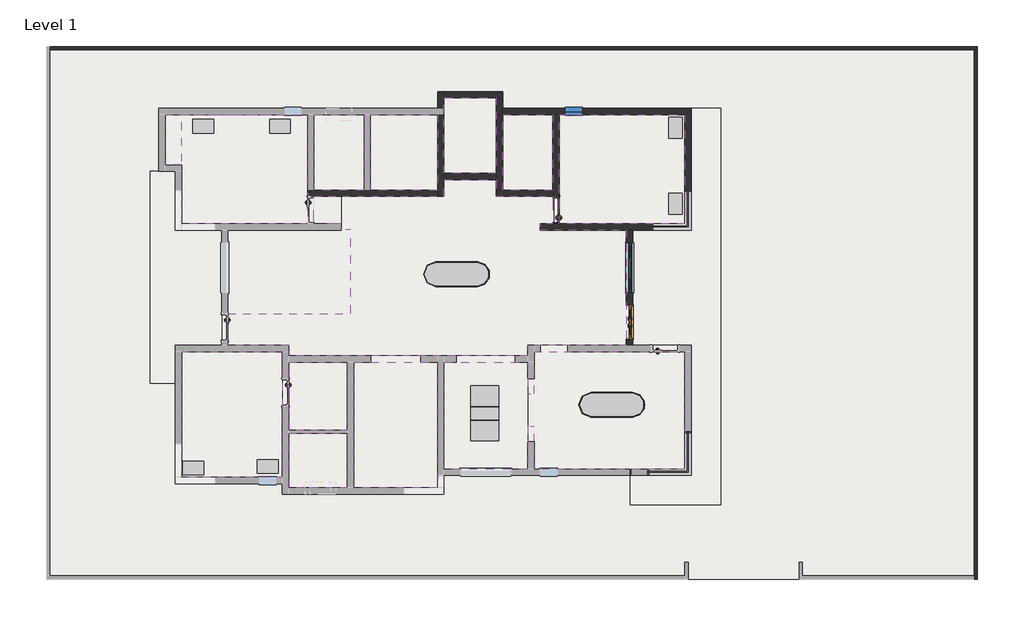
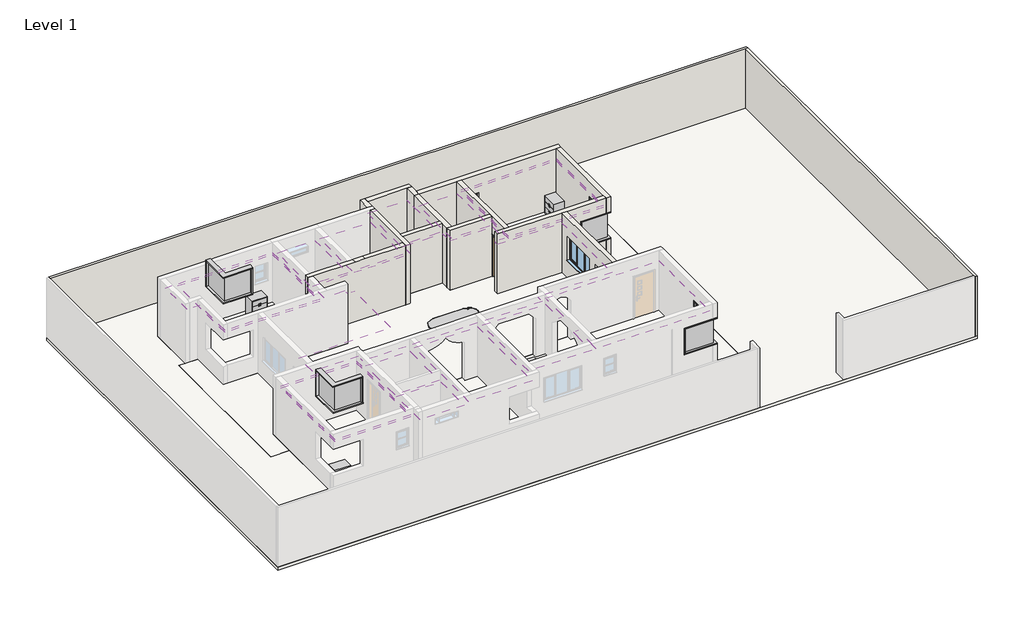
# One storey, part 2 of 2: 15 coverings, 15 slabs, 15 walls, 9 furniture elements, 2 doors, 2 windows, 1 proxy.
"""IFC4 building model written with IfcOpenShell, lengths in millimetres."""

from ifc_helpers import new_model, si_unit, point, frame, frame_2d, origin, origin_with_axes, place, context, project, spatial, polyline, circle_curve, trimmed, segment, composite_curve, outline, extrude, faceted_brep, transform, mapped, element, save
from components import generic_models_1_generic_models_1_b24af07e, door_6c7b9bf3, door_cca51ba5, furniture_cabinet_file_lateral_3_drawer_760_x_500_x_915mm_92c95d2d, furniture_cabinet_file_lateral_3_drawer_760_x_500_x_915mm_e725971a, furniture_table_dining_elliptical_glass_2400x900x720mm_3aac8a2d, furniture_table_dining_w_chairs_rectangular_2000x1000x750mm_b8cbee69, windows_sgl_swept_head_window_2_x3_cc7253b0, windows_tpl_plain_window_6_x4_c25596e0

model = new_model("IFC4")

# Units and contexts
model_context = context("Model", 3, world=origin())
ifc_project = project(units=[si_unit("LENGTHUNIT", "METRE", prefix="MILLI")], contexts=[model_context])

# Site, building, storey
site = spatial("IfcSite", under=ifc_project)
building = spatial("IfcBuilding", under=site)
storey = spatial("IfcBuildingStorey", under=building, Name="Level 1", Elevation=0.0)

# Proxy
placement = place(None, origin())
generic_models_1_generic_models_1_shape = generic_models_1_generic_models_1_b24af07e(model_context)
element("IfcBuildingElementProxy", 1, Name="Generic Models 1 : Generic Models 1", ObjectType="Generic Models 1 : Generic Models 1", at=placement, inside=storey, context=model_context, shape_type="MappedRepresentation", body=[
    mapped(generic_models_1_generic_models_1_shape, transform((0.0, 0.0, 0.0), x_axis=(1.0, 0.0, 0.0), y_axis=(0.0, 1.0, 0.0), z_axis=(0.0, 0.0, 1.0))),
])

# Coverings
element("IfcCovering", 2, ObjectType="2' x 4' ACT System", at=placement, inside=storey, context=model_context, shape_type="SweptSolid", body=[
    extrude(outline(polyline([(2650.3621497, 5508.7135417), (2650.3621497, 7756.6135417), (2650.3621497, 8251.9135417), (4555.3621497, 8251.9135417), (4555.3621497, 7756.6135417), (4555.3621497, 5508.7135417), (2650.3621497, 5508.7135417)])), frame((0.0, 0.0, 2438.4), z_axis=(0.0, 0.0, 1.0), x_axis=(1.0, 0.0, 0.0)), (0.0, 0.0, 1.0), 57.15),
])
element("IfcCovering", 3, ObjectType="2' x 4' ACT System", at=placement, inside=storey, context=model_context, shape_type="SweptSolid", body=[
    extrude(outline(polyline([(-16.6378503, 4899.1135417), (-16.6378503, 7642.3135417), (2421.7621497, 7642.3135417), (2421.7621497, 4899.1135417), (-16.6378503, 4899.1135417)])), frame((0.0, 0.0, 2438.4), z_axis=(0.0, 0.0, 1.0), x_axis=(1.0, 0.0, 0.0)), (0.0, 0.0, 1.0), 57.15),
])
element("IfcCovering", 4, ObjectType="2' x 4' ACT System", at=placement, inside=storey, context=model_context, shape_type="SweptSolid", body=[
    extrude(outline(polyline([(-2074.0378503, 7642.3135417), (-245.2378503, 7642.3135417), (-245.2378503, 4899.1135417), (-2074.0378503, 4899.1135417), (-2074.0378503, 7642.3135417)])), frame((0.0, 0.0, 2438.4), z_axis=(0.0, 0.0, 1.0), x_axis=(1.0, 0.0, 0.0)), (0.0, 0.0, 1.0), 57.15),
])
element("IfcCovering", 5, ObjectType="2' x 4' ACT System", at=placement, inside=storey, context=model_context, shape_type="SweptSolid", body=[
    extrude(outline(polyline([(4783.9621497, 7642.3135417), (6612.7621497, 7642.3135417), (6612.7621497, 4899.1135417), (4783.9621497, 4899.1135417), (4783.9621497, 7642.3135417)])), frame((0.0, 0.0, 2438.4), z_axis=(0.0, 0.0, 1.0), x_axis=(1.0, 0.0, 0.0)), (0.0, 0.0, 1.0), 57.15),
])
element("IfcCovering", 6, ObjectType="2' x 4' ACT System", at=placement, inside=storey, context=model_context, shape_type="SweptSolid", body=[
    extrude(outline(polyline([(-854.8378503, -5921.3648645), (-2988.4378503, -5921.3648645), (-2988.4378503, -3940.1648645), (-854.8378503, -3940.1648645), (-854.8378503, -5921.3648645)])), frame((0.0, 0.0, 2438.4), z_axis=(0.0, 0.0, 1.0), x_axis=(1.0, 0.0, 0.0)), (0.0, 0.0, 1.0), 57.15),
])
element("IfcCovering", 7, ObjectType="2' x 4' ACT System", at=placement, inside=storey, context=model_context, shape_type="SweptSolid", body=[
    extrude(outline(polyline([(-854.8378503, -3825.8648645), (-2988.4378503, -3825.8648645), (-2988.4378503, -1349.2864583), (-854.8378503, -1349.2864583), (-854.8378503, -3825.8648645)])), frame((0.0, 0.0, 2438.4), z_axis=(0.0, 0.0, 1.0), x_axis=(1.0, 0.0, 0.0)), (0.0, 0.0, 1.0), 57.15),
])
element("IfcCovering", 8, ObjectType="2' x 4' ACT System", at=placement, inside=storey, context=model_context, shape_type="SweptSolid", body=[
    extrude(outline(polyline([(-6874.6378503, 7642.3135417), (-2302.6378503, 7642.3135417), (-2302.6378503, 3679.9135417), (-6874.6378503, 3679.9135417), (-6874.6378503, 7642.3135417)]), holes=[polyline([(-2328.0378503, 3705.3135417), (-2328.0378503, 7616.9135417), (-6849.2378503, 7616.9135417), (-6849.2378503, 3705.3135417), (-2328.0378503, 3705.3135417)])]), frame((0.0, 0.0, 2438.4), z_axis=(0.0, 0.0, 1.0), x_axis=(1.0, 0.0, 0.0)), (0.0, 0.0, 1.0), 57.15),
    extrude(outline(polyline([(-2785.2378503, 7159.7135417), (-2785.2378503, 4162.5135417), (-6392.0378503, 4162.5135417), (-6392.0378503, 7159.7135417), (-2785.2378503, 7159.7135417)]), holes=[polyline([(-4004.4378503, 6894.4913463), (-6163.98977, 6894.4913463), (-6163.98977, 6742.0913463), (-4004.4378503, 6742.0913463), (-4004.4378503, 6894.4913463)]), polyline([(-6163.98977, 6132.4913463), (-4004.4378503, 6132.4913463), (-4004.4378503, 6284.8913463), (-6163.98977, 6284.8913463), (-6163.98977, 6132.4913463)]), polyline([(-6163.98977, 5522.8913463), (-4004.4378503, 5522.8913463), (-4004.4378503, 5675.2913463), (-6163.98977, 5675.2913463), (-6163.98977, 5522.8913463)]), polyline([(-4004.4378503, 5065.6913463), (-6163.98977, 5065.6913463), (-6163.98977, 4913.2913463), (-4004.4378503, 4913.2913463), (-4004.4378503, 5065.6913463)]), polyline([(-6163.98977, 4303.6913463), (-4004.4378503, 4303.6913463), (-4004.4378503, 4456.0913463), (-6163.98977, 4456.0913463), (-6163.98977, 4303.6913463)]), polyline([(-3030.6104305, 6580.7706086), (-3693.5284061, 6580.7706086), (-3693.5284061, 6132.4913463), (-3030.6104305, 6132.4913463), (-3030.6104305, 6580.7706086)]), polyline([(-3030.6104305, 5254.9346574), (-3693.5284061, 5254.9346574), (-3693.5284061, 4757.7461757), (-3030.6104305, 4757.7461757), (-3030.6104305, 5254.9346574)])]), frame((0.0, 0.0, 2438.4), z_axis=(0.0, 0.0, 1.0), x_axis=(1.0, 0.0, 0.0)), (0.0, 0.0, 1.0), 57.15),
])
element("IfcCovering", 9, ObjectType="2' x 4' ACT System", at=placement, inside=storey, context=model_context, shape_type="SweptSolid", body=[
    extrude(outline(polyline([(-7484.2378503, 5813.5135417), (-7484.2378503, 7642.3135417), (-2302.6378503, 7642.3135417), (-2302.6378503, 4784.8135417), (-2302.6378503, 3679.9135417), (-6874.6378503, 3679.9135417), (-6874.6378503, 5813.5135417), (-7484.2378503, 5813.5135417)])), frame((0.0, 0.0, 2540.0), z_axis=(0.0, 0.0, 1.0), x_axis=(1.0, 0.0, 0.0)), (0.0, 0.0, 1.0), 57.15),
])
element("IfcCovering", 10, ObjectType="2' x 4' ACT System", at=placement, inside=storey, context=model_context, shape_type="SweptSolid", body=[
    extrude(outline(polyline([(11413.3621497, 7642.3135417), (11413.3621497, 3679.9135417), (6841.3621497, 3679.9135417), (6841.3621497, 7642.3135417), (11413.3621497, 7642.3135417)]), holes=[polyline([(11387.9621497, 3705.3135417), (11387.9621497, 7616.9135417), (6866.7621497, 7616.9135417), (6866.7621497, 3705.3135417), (11387.9621497, 3705.3135417)])]), frame((0.0, 0.0, 2438.4), z_axis=(0.0, 0.0, 1.0), x_axis=(1.0, 0.0, 0.0)), (0.0, 0.0, 1.0), 57.15),
    extrude(outline(polyline([(10930.7621497, 4162.5135417), (7323.9621497, 4162.5135417), (7323.9621497, 7159.7135417), (10930.7621497, 7159.7135417), (10930.7621497, 4162.5135417)]), holes=[composite_curve([segment(trimmed(circle_curve(frame_2d((9059.473925, 5744.3671028)), 1162.7055125), [point((7896.7684125, 5744.3671028))], [point((10222.1794374, 5744.3671028))], True, "CARTESIAN"), True, "CONTINUOUS"), segment(trimmed(circle_curve(frame_2d((9059.473925, 5744.3671028)), 1162.7055125), [point((10222.1794374, 5744.3671028))], [point((7896.7684125, 5744.3671028))], True, "CARTESIAN"), True, "CONTINUOUS")], self_intersect=False), polyline([(10632.4854084, 6840.2533812), (10175.2854084, 6840.2533812), (10175.2854084, 6535.4533812), (10632.4854084, 6535.4533812), (10632.4854084, 6840.2533812)]), polyline([(7913.7746339, 6840.2533812), (7535.1957378, 6840.2533812), (7535.1957378, 6535.4533812), (7913.7746339, 6535.4533812), (7913.7746339, 6840.2533812)]), polyline([(7913.7746339, 4670.5135417), (7535.1957378, 4670.5135417), (7535.1957378, 4439.2661712), (7913.7746339, 4439.2661712), (7913.7746339, 4670.5135417)]), polyline([(10632.4854084, 4670.5135417), (10175.2854084, 4670.5135417), (10175.2854084, 4439.2661712), (10632.4854084, 4439.2661712), (10632.4854084, 4670.5135417)])]), frame((0.0, 0.0, 2438.4), z_axis=(0.0, 0.0, 1.0), x_axis=(1.0, 0.0, 0.0)), (0.0, 0.0, 1.0), 57.15),
])
element("IfcCovering", 11, ObjectType="2' x 4' ACT System", at=placement, inside=storey, context=model_context, shape_type="SweptSolid", body=[
    extrude(outline(polyline([(6841.3621497, 3679.9135417), (6841.3621497, 7642.3135417), (11413.3621497, 7642.3135417), (11413.3621497, 3679.9135417), (6841.3621497, 3679.9135417)])), frame((0.0, 0.0, 2540.0), z_axis=(0.0, 0.0, 1.0), x_axis=(1.0, 0.0, 0.0)), (0.0, 0.0, 1.0), 57.15),
])
element("IfcCovering", 12, ObjectType="2' x 4' ACT System", at=placement, inside=storey, context=model_context, shape_type="SweptSolid", body=[
    extrude(outline(polyline([(6612.7621497, 3679.9135417), (6155.5621497, 3679.9135417), (6155.5621497, 3451.3135417), (9279.7621497, 3451.3135417), (9279.7621497, -739.6864583), (5698.3621497, -739.6864583), (5698.3621497, -1120.6864583), (2536.0621497, -1120.6864583), (-2988.4378503, -1120.6864583), (-2988.4378503, -739.6864583), (-5197.7457903, -739.6864583), (-5197.7457903, 416.1965995), (-740.5378503, 416.1965995), (-740.5378503, 3451.3135417), (-1083.4378503, 3451.3135417), (-1083.4378503, 3679.9135417), (-2074.0378503, 3679.9135417), (-2074.0378503, 4670.5135417), (2650.3621497, 4670.5135417), (2650.3621497, 5280.1135417), (4555.3621497, 5280.1135417), (4555.3621497, 4670.5135417), (6612.7621497, 4670.5135417), (6612.7621497, 3679.9135417)])), frame((0.0, 0.0, 2540.0), z_axis=(0.0, 0.0, 1.0), x_axis=(1.0, 0.0, 0.0)), (0.0, 0.0, 1.0), 57.15),
])
element("IfcCovering", 13, ObjectType="2' x 4' ACT System", at=placement, inside=storey, context=model_context, shape_type="SweptSolid", body=[
    extrude(outline(polyline([(2650.3621497, -5235.4864583), (2650.3621497, -1349.2864583), (5698.3621497, -1349.2864583), (5698.3621497, -2498.0526208), (5926.9621497, -2498.0526208), (5926.9621497, -1234.9864583), (5926.9621497, -968.2864583), (11413.3621497, -968.2864583), (11413.3621497, -5235.4864583), (5926.9621497, -5235.4864583), (5926.9621497, -3706.1656535), (5698.3621497, -3706.1656535), (5698.3621497, -5235.4864583), (2650.3621497, -5235.4864583)])), frame((0.0, 0.0, 2540.0), z_axis=(0.0, 0.0, 1.0), x_axis=(1.0, 0.0, 0.0)), (0.0, 0.0, 1.0), 57.15),
])
element("IfcCovering", 14, ObjectType="2' x 4' ACT System", at=placement, inside=storey, context=model_context, shape_type="SweptSolid", body=[
    extrude(outline(polyline([(2421.7621497, -1349.2864583), (2421.7621497, -5921.3648645), (-626.2378503, -5921.3648645), (-626.2378503, -1349.2864583), (2421.7621497, -1349.2864583)])), frame((0.0, 0.0, 2540.0), z_axis=(0.0, 0.0, 1.0), x_axis=(1.0, 0.0, 0.0)), (0.0, 0.0, 1.0), 57.15),
])
element("IfcCovering", 15, ObjectType="2' x 4' ACT System", at=placement, inside=storey, context=model_context, shape_type="SweptSolid", body=[
    extrude(outline(polyline([(-3217.0378503, -968.2864583), (-3217.0378503, -5540.2864583), (-6874.6378503, -5540.2864583), (-6874.6378503, -968.2864583), (-3217.0378503, -968.2864583)]), holes=[polyline([(-3242.4378503, -5514.8864583), (-3242.4378503, -993.6864583), (-6849.2378503, -993.6864583), (-6849.2378503, -5514.8864583), (-3242.4378503, -5514.8864583)])]), frame((0.0, 0.0, 2438.4), z_axis=(0.0, 0.0, 1.0), x_axis=(1.0, 0.0, 0.0)), (0.0, 0.0, 1.0), 57.15),
    extrude(outline(polyline([(-3699.6378503, -5057.6864583), (-6392.0378503, -5057.6864583), (-6392.0378503, -1450.8864583), (-3699.6378503, -1450.8864583), (-3699.6378503, -5057.6864583)]), holes=[composite_curve([segment(trimmed(circle_curve(frame_2d((-4378.7217073, -3267.5956414)), 304.8), [point((-4683.5217073, -3267.5956414))], [point((-4073.9217073, -3267.5956414))], True, "CARTESIAN"), True, "CONTINUOUS"), segment(trimmed(circle_curve(frame_2d((-4378.7217073, -3267.5956414)), 304.8), [point((-4073.9217073, -3267.5956414))], [point((-4683.5217073, -3267.5956414))], True, "CARTESIAN"), True, "CONTINUOUS")], self_intersect=False), composite_curve([segment(trimmed(circle_curve(frame_2d((-4479.9101454, -2141.3883987)), 609.6), [point((-5089.5101454, -2141.3883987))], [point((-3870.3101454, -2141.3883987))], True, "CARTESIAN"), True, "CONTINUOUS"), segment(trimmed(circle_curve(frame_2d((-4479.9101454, -2141.3883987)), 609.6), [point((-3870.3101454, -2141.3883987))], [point((-5089.5101454, -2141.3883987))], True, "CARTESIAN"), True, "CONTINUOUS")], self_intersect=False), composite_curve([segment(trimmed(circle_curve(frame_2d((-4470.068217, -4339.4664965)), 609.6), [point((-5079.668217, -4339.4664965))], [point((-3860.468217, -4339.4664965))], True, "CARTESIAN"), True, "CONTINUOUS"), segment(trimmed(circle_curve(frame_2d((-4470.068217, -4339.4664965)), 609.6), [point((-3860.468217, -4339.4664965))], [point((-5079.668217, -4339.4664965))], True, "CARTESIAN"), True, "CONTINUOUS")], self_intersect=False), polyline([(-6088.895224, -1599.1474301), (-6241.295224, -1599.1474301), (-6241.295224, -4951.9474301), (-6088.895224, -4951.9474301), (-6088.895224, -1599.1474301)]), polyline([(-5756.1597964, -1599.1474301), (-5920.7593165, -1599.1474301), (-5920.7593165, -4951.9474301), (-5756.1597964, -4951.9474301), (-5756.1597964, -1599.1474301)]), polyline([(-5409.634491, -1599.1474301), (-5574.234011, -1599.1474301), (-5574.234011, -4951.9474301), (-5409.634491, -4951.9474301), (-5409.634491, -1599.1474301)])]), frame((0.0, 0.0, 2438.4), z_axis=(0.0, 0.0, 1.0), x_axis=(1.0, 0.0, 0.0)), (0.0, 0.0, 1.0), 57.15),
])
element("IfcCovering", 16, ObjectType="2' x 4' ACT System", at=placement, inside=storey, context=model_context, shape_type="SweptSolid", body=[
    extrude(outline(polyline([(-6874.6378503, -968.2864583), (-3217.0378503, -968.2864583), (-3217.0378503, -5540.2864583), (-6874.6378503, -5540.2864583), (-6874.6378503, -968.2864583)])), frame((0.0, 0.0, 2540.0), z_axis=(0.0, 0.0, 1.0), x_axis=(1.0, 0.0, 0.0)), (0.0, 0.0, 1.0), 57.15),
])

# Doors
door_shape = door_6c7b9bf3(model_context)
element("IfcDoor", 17, ObjectType="Doors_ExtDbl_Louvre : External Door 4'X7\"", at=placement, inside=storey, context=model_context, shape_type="MappedRepresentation", body=[
    mapped(door_shape, transform((9394.0621497, 98.5135417, 0.0), x_axis=(0.0, 1.0, 0.0), y_axis=(-1.0, 0.0, 0.0), z_axis=(0.0, 0.0, 1.0))),
])
door_2_shape = door_cca51ba5(model_context)
element("IfcDoor", 18, ObjectType="Doors_IntSgl_4 : Internal Door 3'3\"X7'", at=placement, inside=storey, context=model_context, shape_type="MappedRepresentation", body=[
    mapped(door_2_shape, transform((6727.0621497, 4175.2135417, 0.0), x_axis=(0.0, 1.0, 0.0), y_axis=(-1.0, 0.0, 0.0), z_axis=(0.0, 0.0, 1.0))),
])

# Furniture
furniture_cabinet_file_lateral_3_drawer_760_x_500_x_915mm_shape = furniture_cabinet_file_lateral_3_drawer_760_x_500_x_915mm_92c95d2d(model_context)
element("IfcFurniture", 19, ObjectType="Furniture_Cabinet_File_Lateral_3-Drawer : 760 x 500 x 915mm", at=placement, inside=storey, context=model_context, shape_type="MappedRepresentation", body=[
    mapped(furniture_cabinet_file_lateral_3_drawer_760_x_500_x_915mm_shape, transform((-3930.4603642, -6080.9048343, 0.0), x_axis=(-1.0, 0.0, 0.0), y_axis=(0.0, -1.0, 0.0), z_axis=(0.0, 0.0, 1.0))),
])
element("IfcFurniture", 20, ObjectType="Furniture_Cabinet_File_Lateral_3-Drawer : 760 x 500 x 915mm", at=placement, inside=storey, context=model_context, shape_type="MappedRepresentation", body=[
    mapped(furniture_cabinet_file_lateral_3_drawer_760_x_500_x_915mm_shape, transform((-6635.5603642, -6131.7048343, 0.0), x_axis=(-1.0, 0.0, 0.0), y_axis=(0.0, -1.0, 0.0), z_axis=(0.0, 0.0, 1.0))),
])
element("IfcFurniture", 21, ObjectType="Furniture_Cabinet_File_Lateral_3-Drawer : 760 x 500 x 915mm", at=placement, inside=storey, context=model_context, shape_type="MappedRepresentation", body=[
    mapped(furniture_cabinet_file_lateral_3_drawer_760_x_500_x_915mm_shape, transform((12004.7805258, 6992.3910278, 0.0), x_axis=(0.0, -1.0, 0.0), y_axis=(1.0, 0.0, 0.0), z_axis=(0.0, 0.0, 1.0))),
])
element("IfcFurniture", 22, ObjectType="Furniture_Cabinet_File_Lateral_3-Drawer : 760 x 500 x 915mm", at=placement, inside=storey, context=model_context, shape_type="MappedRepresentation", body=[
    mapped(furniture_cabinet_file_lateral_3_drawer_760_x_500_x_915mm_shape, transform((12004.7805258, 4223.7910278, 0.0), x_axis=(0.0, -1.0, 0.0), y_axis=(1.0, 0.0, 0.0), z_axis=(0.0, 0.0, 1.0))),
])
furniture_cabinet_file_lateral_3_drawer_760_x_500_x_915mm_2_shape = furniture_cabinet_file_lateral_3_drawer_760_x_500_x_915mm_e725971a(model_context)
element("IfcFurniture", 23, ObjectType="Furniture_Cabinet_File_Lateral_3-Drawer : 760 x 500 x 915mm", at=placement, inside=storey, context=model_context, shape_type="MappedRepresentation", body=[
    mapped(furniture_cabinet_file_lateral_3_drawer_760_x_500_x_915mm_2_shape, transform((-6279.9603642, 8157.5319178, 0.0), x_axis=(-1.0, 0.0, 0.0), y_axis=(0.0, -1.0, 0.0), z_axis=(0.0, 0.0, 1.0))),
])
element("IfcFurniture", 24, ObjectType="Furniture_Cabinet_File_Lateral_3-Drawer : 760 x 500 x 915mm", at=placement, inside=storey, context=model_context, shape_type="MappedRepresentation", body=[
    mapped(furniture_cabinet_file_lateral_3_drawer_760_x_500_x_915mm_2_shape, transform((-3485.4683042, 8157.5319178, 0.0), x_axis=(-1.0, 0.0, 0.0), y_axis=(0.0, -1.0, 0.0), z_axis=(0.0, 0.0, 1.0))),
])
furniture_table_dining_elliptical_glass_2400x900x720mm_shape = furniture_table_dining_elliptical_glass_2400x900x720mm_3aac8a2d(model_context)
element("IfcFurniture", 25, ObjectType="Furniture_Table_Dining_Elliptical : Glass-2400x900x720mm", at=placement, inside=storey, context=model_context, shape_type="MappedRepresentation", body=[
    mapped(furniture_table_dining_elliptical_glass_2400x900x720mm_shape, transform((9154.6818218, -2546.0880976, 0.0), x_axis=(1.0, 0.0, 0.0), y_axis=(0.0, 1.0, 0.0), z_axis=(0.0, 0.0, 1.0))),
])
element("IfcFurniture", 26, ObjectType="Furniture_Table_Dining_Elliptical : Glass-2400x900x720mm", at=placement, inside=storey, context=model_context, shape_type="MappedRepresentation", body=[
    mapped(furniture_table_dining_elliptical_glass_2400x900x720mm_shape, transform((3515.8818218, 2203.7119024, 0.0), x_axis=(1.0, 0.0, 0.0), y_axis=(0.0, 1.0, 0.0), z_axis=(0.0, 0.0, 1.0))),
])
furniture_table_dining_w_chairs_rectangular_2000x1000x750mm_shape = furniture_table_dining_w_chairs_rectangular_2000x1000x750mm_b8cbee69(model_context)
element("IfcFurniture", 27, ObjectType="Furniture_Table_Dining_w-Chairs_Rectangular : 2000x1000x750mm_w-4_Seats", at=placement, inside=storey, context=model_context, shape_type="MappedRepresentation", body=[
    mapped(furniture_table_dining_w_chairs_rectangular_2000x1000x750mm_shape, transform((4180.6167789, -3334.3651801, 0.0), x_axis=(0.0, 1.0, 0.0), y_axis=(-1.0, 0.0, 0.0), z_axis=(0.0, 0.0, 1.0))),
])

# Slabs
element("IfcSlab", 28, ObjectType="Generic - 6\"", at=placement, inside=storey, context=model_context, shape_type="SweptSolid", body=[
    extrude(outline(polyline([(6640.7435765, 7870.9135417), (11641.9621497, 7870.9135417), (11641.9621497, 3451.3135417), (6640.7435765, 3451.3135417), (6640.7435765, 7870.9135417)])), frame((0.0, 0.0, -152.4), z_axis=(0.0, 0.0, 1.0), x_axis=(1.0, 0.0, 0.0)), (0.0, 0.0, 1.0), 152.4),
])
element("IfcSlab", 29, ObjectType="Generic - 6\"", at=placement, inside=storey, context=model_context, shape_type="SweptSolid", body=[
    extrude(outline(polyline([(4555.3621497, 7870.9135417), (6640.7435765, 7870.9135417), (6640.7435765, 4670.5135417), (4555.3621497, 4670.5135417), (4555.3621497, 7870.9135417)])), frame((0.0, 0.0, -152.4), z_axis=(0.0, 0.0, 1.0), x_axis=(1.0, 0.0, 0.0)), (0.0, 0.0, 1.0), 152.4),
])
element("IfcSlab", 30, ObjectType="Generic - 6\"", at=placement, inside=storey, context=model_context, shape_type="SweptSolid", body=[
    extrude(outline(polyline([(4783.9621497, 7870.9135417), (4555.3621497, 7870.9135417), (4555.3621497, 5280.1135417), (2421.7621497, 5280.1135417), (2421.7621497, 8480.5135417), (4783.9621497, 8480.5135417), (4783.9621497, 7870.9135417)])), frame((0.0, 0.0, -152.4), z_axis=(0.0, 0.0, 1.0), x_axis=(1.0, 0.0, 0.0)), (0.0, 0.0, 1.0), 152.4),
])
element("IfcSlab", 31, ObjectType="Generic - 6\"", at=placement, inside=storey, context=model_context, shape_type="SweptSolid", body=[
    extrude(outline(polyline([(-247.4877588, 7870.9135417), (2421.7621497, 7870.9135417), (2421.7621497, 5280.1135417), (2650.3621497, 5280.1135417), (2650.3621497, 4670.5135417), (2421.7621497, 4670.5135417), (-247.4877588, 4670.5135417), (-247.4877588, 7870.9135417)])), frame((0.0, 0.0, -152.4), z_axis=(0.0, 0.0, 1.0), x_axis=(1.0, 0.0, 0.0)), (0.0, 0.0, 1.0), 152.4),
])
element("IfcSlab", 32, ObjectType="Generic - 6\"", at=placement, inside=storey, context=model_context, shape_type="SweptSolid", body=[
    extrude(outline(polyline([(-2302.6378503, 7870.9135417), (-247.4877588, 7870.9135417), (-247.4877588, 4670.5135417), (-2302.6378503, 4670.5135417), (-2302.6378503, 7870.9135417)])), frame((0.0, 0.0, -152.4), z_axis=(0.0, 0.0, 1.0), x_axis=(1.0, 0.0, 0.0)), (0.0, 0.0, 1.0), 152.4),
])
element("IfcSlab", 33, ObjectType="Generic - 6\"", at=placement, inside=storey, context=model_context, shape_type="SweptSolid", body=[
    extrude(outline(polyline([(-7712.8378503, 7870.9135417), (-2302.6378503, 7870.9135417), (-2302.6378503, 4670.5135417), (-1083.4378503, 4670.5135417), (-1083.4378503, 3451.3135417), (-7103.2378503, 3451.3135417), (-7103.2378503, 5584.9135417), (-7712.8378503, 5584.9135417), (-7712.8378503, 7870.9135417)])), frame((0.0, 0.0, -152.4), z_axis=(0.0, 0.0, 1.0), x_axis=(1.0, 0.0, 0.0)), (0.0, 0.0, 1.0), 152.4),
])
element("IfcSlab", 34, ObjectType="Generic - 6\"", at=placement, inside=storey, context=model_context, shape_type="SweptSolid", body=[
    extrude(outline(polyline([(-1083.4378503, 3451.3135417), (-1083.4378503, 4670.5135417), (2650.3621497, 4670.5135417), (2650.3621497, 5280.1135417), (4555.3621497, 5280.1135417), (4555.3621497, 4670.5135417), (6640.7435765, 4670.5135417), (6640.7435765, 3451.3135417), (9508.3621497, 3451.3135417), (9508.3621497, -739.6864583), (5698.3621497, -739.6864583), (5698.3621497, -1120.6864583), (-3217.0378503, -1120.6864583), (-3217.0378503, -739.6864583), (-5426.3457903, -739.6864583), (-5426.3457903, 3451.3135417), (-1083.4378503, 3451.3135417)])), frame((0.0, 0.0, -152.4), z_axis=(0.0, 0.0, 1.0), x_axis=(1.0, 0.0, 0.0)), (0.0, 0.0, 1.0), 152.4),
])
element("IfcSlab", 35, ObjectType="Generic - 6\"", at=placement, inside=storey, context=model_context, shape_type="SweptSolid", body=[
    extrude(outline(polyline([(-3217.0378503, -739.6864583), (-3217.0378503, -5768.8864583), (-7103.2378503, -5768.8864583), (-7103.2378503, -739.6864583), (-3217.0378503, -739.6864583)])), frame((0.0, 0.0, -152.4), z_axis=(0.0, 0.0, 1.0), x_axis=(1.0, 0.0, 0.0)), (0.0, 0.0, 1.0), 152.4),
])
element("IfcSlab", 36, ObjectType="Generic - 6\"", at=placement, inside=storey, context=model_context, shape_type="SweptSolid", body=[
    extrude(outline(polyline([(-739.1672564, -1120.6864583), (-739.1672564, -6149.9648645), (-3217.0378503, -6149.9648645), (-3217.0378503, -1120.6864583), (-739.1672564, -1120.6864583)])), frame((0.0, 0.0, -152.4), z_axis=(0.0, 0.0, 1.0), x_axis=(1.0, 0.0, 0.0)), (0.0, 0.0, 1.0), 152.4),
])
element("IfcSlab", 37, ObjectType="Generic - 6\"", at=placement, inside=storey, context=model_context, shape_type="SweptSolid", body=[
    extrude(outline(polyline([(2650.3621497, -1120.6864583), (2650.3621497, -6149.9648645), (-739.1672564, -6149.9648645), (-739.1672564, -1120.6864583), (2650.3621497, -1120.6864583)])), frame((0.0, 0.0, -152.4), z_axis=(0.0, 0.0, 1.0), x_axis=(1.0, 0.0, 0.0)), (0.0, 0.0, 1.0), 152.4),
])
element("IfcSlab", 38, ObjectType="Generic - 6\"", at=placement, inside=storey, context=model_context, shape_type="SweptSolid", body=[
    extrude(outline(polyline([(2650.3621497, -1120.6864583), (5698.3621497, -1120.6864583), (5698.3621497, -5464.0864583), (2650.3621497, -5464.0864583), (2650.3621497, -1120.6864583)])), frame((0.0, 0.0, -152.4), z_axis=(0.0, 0.0, 1.0), x_axis=(1.0, 0.0, 0.0)), (0.0, 0.0, 1.0), 152.4),
])
element("IfcSlab", 39, ObjectType="Generic - 6\"", at=placement, inside=storey, context=model_context, shape_type="SweptSolid", body=[
    extrude(outline(polyline([(11641.9621497, -739.6864583), (11641.9621497, -5464.0864583), (5698.3621497, -5464.0864583), (5698.3621497, -739.6864583), (11641.9621497, -739.6864583)])), frame((0.0, 0.0, -152.4), z_axis=(0.0, 0.0, 1.0), x_axis=(1.0, 0.0, 0.0)), (0.0, 0.0, 1.0), 152.4),
])
element("IfcSlab", 40, ObjectType="Generic - 6\"", at=placement, inside=storey, context=model_context, shape_type="SweptSolid", body=[
    extrude(outline(polyline([(12708.7621497, 7870.9135417), (12708.7621497, -6531.2666852), (9432.1621497, -6531.2666852), (9432.1621497, -5464.0864583), (11641.9621497, -5464.0864583), (11641.9621497, -739.6864583), (9508.3621497, -739.6864583), (9508.3621497, 3451.3135417), (11641.9621497, 3451.3135417), (11641.9621497, 7870.9135417), (12708.7621497, 7870.9135417)])), frame((0.0, 0.0, -152.4), z_axis=(0.0, 0.0, 1.0), x_axis=(1.0, 0.0, 0.0)), (0.0, 0.0, 1.0), 152.4),
])
element("IfcSlab", 41, ObjectType="Generic - 6\"", at=placement, inside=storey, context=model_context, shape_type="SweptSolid", body=[
    extrude(outline(polyline([(-8017.6378503, 5584.9135417), (-7103.2378503, 5584.9135417), (-7103.2378503, 3451.3135417), (-5426.3457903, 3451.3135417), (-5426.3457903, -739.6864583), (-7103.2378503, -739.6864583), (-7103.2378503, -2111.2864583), (-8017.6378503, -2111.2864583), (-8017.6378503, 5584.9135417)])), frame((0.0, 0.0, -152.4), z_axis=(0.0, 0.0, 1.0), x_axis=(1.0, 0.0, 0.0)), (0.0, 0.0, 1.0), 152.4),
])
element("IfcSlab", 42, ObjectType="Generic - 6\" 2", at=placement, inside=storey, context=model_context, shape_type="SweptSolid", body=[
    extrude(outline(polyline([(22043.2621497, 10118.8135417), (22043.2621497, -9235.9864583), (-11789.5378503, -9235.9864583), (-11789.5378503, 10118.8135417), (22043.2621497, 10118.8135417)]), holes=[polyline([(2650.3621497, -5464.0864583), (9432.1621497, -5464.0864583), (9432.1621497, -6531.2666852), (12708.7621497, -6531.2666852), (12708.7621497, 7870.9135417), (4783.9621497, 7870.9135417), (4783.9621497, 8480.5135417), (2421.7621497, 8480.5135417), (2421.7621497, 7870.9135417), (-7712.8378503, 7870.9135417), (-7712.8378503, 5584.9135417), (-8017.6378503, 5584.9135417), (-8017.6378503, -2111.2864583), (-7103.2378503, -2111.2864583), (-7103.2378503, -5768.8864583), (-3217.0378503, -5768.8864583), (-3217.0378503, -6149.9648645), (2650.3621497, -6149.9648645), (2650.3621497, -5464.0864583)])]), frame((0.0, 0.0, -152.4), z_axis=(0.0, 0.0, 1.0), x_axis=(1.0, 0.0, 0.0)), (0.0, 0.0, 1.0), 152.4),
])

# Walls
element("IfcWall", 43, ObjectType="Generic - 4.5\"", at=placement, inside=storey, context=model_context, shape_type="Brep", body=[
    faceted_brep([(-11675.2378503, 10004.5135417, 0.0), (21928.9621497, 10004.5135417, 0.0), (22043.2621497, 10004.5135417, 0.0), (22043.2621497, 10004.5135417, 3048.0), (21928.9621497, 10004.5135417, 3048.0), (-11675.2378503, 10004.5135417, 3048.0), (-11675.2378503, 10118.8135417, 0.0), (-11675.2378503, 10118.8135417, 3048.0), (22043.2621497, 10118.8135417, 3048.0), (22043.2621497, 10118.8135417, 0.0)], [[[0, 1, 2, 3, 4, 5]], [[6, 7, 8, 9]], [[2, 1, 0, 6, 9]], [[5, 4, 3, 8, 7]], [[0, 5, 7, 6]], [[3, 2, 9, 8]]]),
])
element("IfcWall", 44, ObjectType="Generic - 4.5\"", at=placement, inside=storey, context=model_context, shape_type="Brep", body=[
    faceted_brep([(21928.9621497, 10004.5135417, 0.0), (21928.9621497, -9121.6864583, 0.0), (21928.9621497, -9235.9864583, 0.0), (21928.9621497, -9235.9864583, 3048.0), (21928.9621497, -9121.6864583, 3048.0), (21928.9621497, 10004.5135417, 3048.0), (22043.2621497, 10004.5135417, 0.0), (22043.2621497, 10004.5135417, 3048.0), (22043.2621497, -9235.9864583, 3048.0), (22043.2621497, -9235.9864583, 0.0)], [[[0, 1, 2, 3, 4, 5]], [[6, 7, 8, 9]], [[2, 1, 0, 6, 9]], [[5, 4, 3, 8, 7]], [[0, 5, 7, 6]], [[3, 2, 9, 8]]]),
])
element("IfcWall", 45, ObjectType="Generic - 9\"", at=placement, inside=storey, context=model_context, shape_type="Brep", body=[
    faceted_brep([(2650.3621497, 7870.9135417, 0.0), (2650.3621497, 8251.9135417, 0.0), (2650.3621497, 8480.5135417, 0.0), (2650.3621497, 8480.5135417, 3048.0), (2650.3621497, 8251.9135417, 3048.0), (2650.3621497, 7870.9135417, 3048.0), (2421.7621497, 7870.9135417, 0.0), (2421.7621497, 7870.9135417, 3048.0), (2421.7621497, 8480.5135417, 3048.0), (2421.7621497, 8480.5135417, 0.0)], [[[0, 1, 2, 3, 4, 5]], [[6, 7, 8, 9]], [[2, 1, 0, 6, 9]], [[0, 5, 7, 6]], [[3, 2, 9, 8]], [[5, 4, 3, 8, 7]]]),
])
element("IfcWall", 46, ObjectType="Generic - 9\"", at=placement, inside=storey, context=model_context, shape_type="Brep", body=[
    faceted_brep([(2650.3621497, 8251.9135417, 0.0), (4555.3621497, 8251.9135417, 0.0), (4783.9621497, 8251.9135417, 0.0), (4783.9621497, 8251.9135417, 3048.0), (4555.3621497, 8251.9135417, 3048.0), (2650.3621497, 8251.9135417, 3048.0), (2650.3621497, 8480.5135417, 0.0), (2650.3621497, 8480.5135417, 3048.0), (4783.9621497, 8480.5135417, 3048.0), (4783.9621497, 8480.5135417, 0.0)], [[[0, 1, 2, 3, 4, 5]], [[6, 7, 8, 9]], [[2, 1, 0, 6, 9]], [[0, 5, 7, 6]], [[3, 2, 9, 8]], [[5, 4, 3, 8, 7]]]),
])
element("IfcWall", 47, ObjectType="Generic - 9\"", at=placement, inside=storey, context=model_context, shape_type="Brep", body=[
    faceted_brep([(4555.3621497, 8251.9135417, 0.0), (4555.3621497, 7642.3135417, 0.0), (4555.3621497, 7642.3135417, 3048.0), (4555.3621497, 8251.9135417, 3048.0), (4783.9621497, 8251.9135417, 0.0), (4783.9621497, 8251.9135417, 3048.0), (4783.9621497, 7870.9135417, 3048.0), (4783.9621497, 7642.3135417, 3048.0), (4783.9621497, 7642.3135417, 0.0), (4783.9621497, 7870.9135417, 0.0)], [[[0, 1, 2, 3]], [[4, 5, 6, 7, 8, 9]], [[1, 0, 4, 9, 8]], [[0, 3, 5, 4]], [[2, 1, 8, 7]], [[3, 2, 7, 6, 5]]]),
])
element("IfcWall", 48, ObjectType="Generic - 9\"", at=placement, inside=storey, context=model_context, shape_type="Brep", body=[
    faceted_brep([(4783.9621497, 7642.3135417, 0.0), (6612.7621497, 7642.3135417, 0.0), (6841.3621497, 7642.3135417, 0.0), (11413.3621497, 7642.3135417, 0.0), (11641.9621497, 7642.3135417, 0.0), (11641.9621497, 7642.3135417, 3048.0), (11413.3621497, 7642.3135417, 3048.0), (6841.3621497, 7642.3135417, 3048.0), (6612.7621497, 7642.3135417, 3048.0), (4783.9621497, 7642.3135417, 3048.0), (7069.9621497, 7642.3135417, 2110.0), (7679.5621497, 7642.3135417, 2110.0), (7679.5621497, 7642.3135417, 1195.6), (7069.9621497, 7642.3135417, 1195.6), (4783.9621497, 7870.9135417, 0.0), (4783.9621497, 7870.9135417, 3048.0), (11641.9621497, 7870.9135417, 3048.0), (11641.9621497, 7870.9135417, 0.0), (7069.9621497, 7870.9135417, 2110.0), (7069.9621497, 7870.9135417, 1195.6), (7679.5621497, 7870.9135417, 1195.6), (7679.5621497, 7870.9135417, 2110.0)], [[[0, 1, 2, 3, 4, 5, 6, 7, 8, 9], [10, 11, 12, 13]], [[14, 15, 16, 17], [18, 19, 20, 21]], [[4, 3, 2, 1, 0, 14, 17]], [[0, 9, 15, 14]], [[5, 4, 17, 16]], [[19, 18, 10, 13]], [[20, 19, 13, 12]], [[21, 20, 12, 11]], [[18, 21, 11, 10]], [[9, 8, 7, 6, 5, 16, 15]]]),
])
element("IfcWall", 49, ObjectType="Generic - 9\"", at=placement, inside=storey, context=model_context, shape_type="Brep", body=[
    faceted_brep([(11413.3621497, 7642.3135417, 0.0), (11413.3621497, 3679.9135417, 0.0), (11413.3621497, 3451.3135417, 0.0), (11413.3621497, 3451.3135417, 914.4), (11413.3621497, 3679.9135417, 914.4), (11413.3621497, 4916.8520795, 914.4), (11413.3621497, 4916.8520795, 2286.0), (11413.3621497, 3679.9135417, 2286.0), (11413.3621497, 3451.3135417, 2286.0), (11413.3621497, 3451.3135417, 3048.0), (11413.3621497, 3679.9135417, 3048.0), (11413.3621497, 7642.3135417, 3048.0), (11641.9621497, 3451.3135417, 0.0), (11641.9621497, 7642.3135417, 0.0), (11641.9621497, 7642.3135417, 3048.0), (11641.9621497, 3451.3135417, 3048.0), (11641.9621497, 3451.3135417, 2286.0), (11641.9621497, 4916.8520795, 2286.0), (11641.9621497, 4916.8520795, 914.4), (11641.9621497, 3451.3135417, 914.4)], [[[0, 1, 2, 3, 4, 5, 6, 7, 8, 9, 10, 11]], [[12, 13, 14, 15, 16, 17, 18, 19]], [[2, 1, 0, 13, 12]], [[0, 11, 14, 13]], [[11, 10, 9, 15, 14]], [[6, 17, 16, 8, 7]], [[18, 5, 4, 3, 19]], [[17, 6, 5, 18]], [[2, 12, 19, 3]], [[15, 9, 8, 16]]]),
])
element("IfcWall", 50, ObjectType="Generic - 9\"", at=placement, inside=storey, context=model_context, shape_type="Brep", body=[
    faceted_brep([(11413.3621497, 3679.9135417, 0.0), (6155.5621497, 3679.9135417, 0.0), (6155.5621497, 3679.9135417, 3048.0), (6612.7621497, 3679.9135417, 3048.0), (6841.3621497, 3679.9135417, 3048.0), (11413.3621497, 3679.9135417, 3048.0), (11413.3621497, 3679.9135417, 2286.0), (10186.0756044, 3679.9135417, 2286.0), (10186.0756044, 3679.9135417, 914.4), (11413.3621497, 3679.9135417, 914.4), (6155.5621497, 3451.3135417, 0.0), (9279.7621497, 3451.3135417, 0.0), (9508.3621497, 3451.3135417, 0.0), (11413.3621497, 3451.3135417, 0.0), (11413.3621497, 3451.3135417, 914.4), (10186.0756044, 3451.3135417, 914.4), (10186.0756044, 3451.3135417, 2286.0), (11413.3621497, 3451.3135417, 2286.0), (11413.3621497, 3451.3135417, 3048.0), (9508.3621497, 3451.3135417, 3048.0), (9279.7621497, 3451.3135417, 3048.0), (6155.5621497, 3451.3135417, 3048.0)], [[[0, 1, 2, 3, 4, 5, 6, 7, 8, 9]], [[10, 11, 12, 13, 14, 15, 16, 17, 18, 19, 20, 21]], [[1, 0, 13, 12, 11, 10]], [[2, 1, 10, 21]], [[5, 4, 3, 2, 21, 20, 19, 18]], [[16, 7, 6, 17]], [[8, 15, 14, 9]], [[7, 16, 15, 8]], [[5, 18, 17, 6]], [[13, 0, 9, 14]]]),
])
element("IfcWall", 51, ObjectType="Generic - 9\"", at=placement, inside=storey, context=model_context, shape_type="Brep", body=[
    faceted_brep([(6612.7621497, 7642.3135417, 3048.0), (6612.7621497, 7642.3135417, 0.0), (6612.7621497, 4899.1135417, 0.0), (6612.7621497, 4670.5135417, 0.0), (6612.7621497, 4670.5135417, 2133.6), (6612.7621497, 3679.9135417, 2133.6), (6612.7621497, 3679.9135417, 3048.0), (6612.7621497, 4670.5135417, 3048.0), (6612.7621497, 4899.1135417, 3048.0), (6841.3621497, 7642.3135417, 0.0), (6841.3621497, 7642.3135417, 3048.0), (6841.3621497, 3679.9135417, 3048.0), (6841.3621497, 3679.9135417, 2133.6), (6841.3621497, 4670.5135417, 2133.6), (6841.3621497, 4670.5135417, 0.0)], [[[0, 1, 2, 3, 4, 5, 6, 7, 8]], [[9, 10, 11, 12, 13, 14]], [[1, 9, 14, 3, 2]], [[1, 0, 10, 9]], [[11, 6, 5, 12]], [[13, 4, 3, 14]], [[4, 13, 12, 5]], [[0, 8, 7, 6, 11, 10]]]),
])
element("IfcWall", 52, ObjectType="Generic - 9\"", at=placement, inside=storey, context=model_context, shape_type="Brep", body=[
    faceted_brep([(6612.7621497, 4899.1135417, 0.0), (4783.9621497, 4899.1135417, 0.0), (4555.3621497, 4899.1135417, 0.0), (4555.3621497, 4899.1135417, 3048.0), (4783.9621497, 4899.1135417, 3048.0), (6612.7621497, 4899.1135417, 3048.0), (6612.7621497, 4670.5135417, 0.0), (6612.7621497, 4670.5135417, 2133.6), (6612.7621497, 4670.5135417, 3048.0), (4555.3621497, 4670.5135417, 3048.0), (4555.3621497, 4670.5135417, 0.0)], [[[0, 1, 2, 3, 4, 5]], [[6, 7, 8, 9, 10]], [[2, 1, 0, 6, 10]], [[0, 5, 8, 7, 6]], [[3, 2, 10, 9]], [[5, 4, 3, 9, 8]]]),
])
element("IfcWall", 53, ObjectType="Generic - 9\"", at=placement, inside=storey, context=model_context, shape_type="Brep", body=[
    faceted_brep([(4783.9621497, 4899.1135417, 0.0), (4783.9621497, 7642.3135417, 0.0), (4783.9621497, 7642.3135417, 3048.0), (4783.9621497, 4899.1135417, 3048.0), (4555.3621497, 4899.1135417, 0.0), (4555.3621497, 4899.1135417, 3048.0), (4555.3621497, 5280.1135417, 3048.0), (4555.3621497, 5508.7135417, 3048.0), (4555.3621497, 7642.3135417, 3048.0), (4555.3621497, 7642.3135417, 0.0), (4555.3621497, 5508.7135417, 0.0), (4555.3621497, 5280.1135417, 0.0)], [[[0, 1, 2, 3]], [[4, 5, 6, 7, 8, 9, 10, 11]], [[1, 0, 4, 11, 10, 9]], [[0, 3, 5, 4]], [[2, 1, 9, 8]], [[3, 2, 8, 7, 6, 5]]]),
])
element("IfcWall", 54, ObjectType="Generic - 9\"", at=placement, inside=storey, context=model_context, shape_type="Brep", body=[
    faceted_brep([(2421.7621497, 7642.3135417, 0.0), (2421.7621497, 4899.1135417, 0.0), (2421.7621497, 4670.5135417, 0.0), (2421.7621497, 4670.5135417, 3048.0), (2421.7621497, 4899.1135417, 3048.0), (2421.7621497, 7642.3135417, 3048.0), (2650.3621497, 7642.3135417, 0.0), (2650.3621497, 7642.3135417, 3048.0), (2650.3621497, 5508.7135417, 3048.0), (2650.3621497, 5280.1135417, 3048.0), (2650.3621497, 4670.5135417, 3048.0), (2650.3621497, 4670.5135417, 0.0), (2650.3621497, 5280.1135417, 0.0), (2650.3621497, 5508.7135417, 0.0)], [[[0, 1, 2, 3, 4, 5]], [[6, 7, 8, 9, 10, 11, 12, 13]], [[2, 1, 0, 6, 13, 12, 11]], [[0, 5, 7, 6]], [[3, 2, 11, 10]], [[5, 4, 3, 10, 9, 8, 7]]]),
])
element("IfcWall", 55, ObjectType="Generic - 9\"", at=placement, inside=storey, context=model_context, shape_type="SweptSolid", body=[
    extrude(outline(polyline([(4555.3621497, 5280.1135417), (2650.3621497, 5280.1135417), (2650.3621497, 5508.7135417), (4555.3621497, 5508.7135417), (4555.3621497, 5280.1135417)])), origin_with_axes(), (0.0, 0.0, 1.0), 3048.0),
])
element("IfcWall", 56, ObjectType="Generic - 9\"", at=placement, inside=storey, context=model_context, shape_type="Brep", body=[
    faceted_brep([(2421.7621497, 4899.1135417, 0.0), (-16.6378503, 4899.1135417, 0.0), (-245.2378503, 4899.1135417, 0.0), (-2074.0378503, 4899.1135417, 0.0), (-2302.6378503, 4899.1135417, 0.0), (-2302.6378503, 4899.1135417, 3048.0), (-2074.0378503, 4899.1135417, 3048.0), (-245.2378503, 4899.1135417, 3048.0), (-16.6378503, 4899.1135417, 3048.0), (478.6621497, 4899.1135417, 3048.0), (2421.7621497, 4899.1135417, 3048.0), (2421.7621497, 4670.5135417, 0.0), (2421.7621497, 4670.5135417, 3048.0), (478.6621497, 4670.5135417, 3048.0), (-16.6378503, 4670.5135417, 3048.0), (-2074.0378503, 4670.5135417, 3048.0), (-2302.6378503, 4670.5135417, 3048.0), (-2302.6378503, 4670.5135417, 2133.6), (-2302.6378503, 4670.5135417, 0.0)], [[[0, 1, 2, 3, 4, 5, 6, 7, 8, 9, 10]], [[11, 12, 13, 14, 15, 16, 17, 18]], [[4, 3, 2, 1, 0, 11, 18]], [[0, 10, 12, 11]], [[5, 4, 18, 17, 16]], [[10, 9, 13, 12]], [[8, 7, 6, 5, 16, 15, 14]], [[9, 8, 14, 13]]]),
])
element("IfcWall", 57, ObjectType="Generic - 9\"", at=placement, inside=storey, context=model_context, shape_type="SweptSolid", body=[
    extrude(outline(polyline([(3451.3135417, 0.0), (708.1135417, 0.0), (708.1135417, 2133.6), (-511.0864583, 2133.6), (-511.0864583, 0.0), (-739.6864583, 0.0), (-739.6864583, 3048.0), (3451.3135417, 3048.0), (3451.3135417, 0.0)]), holes=[polyline([(2993.5182292, 2110.0), (1164.7182292, 2110.0), (1164.7182292, 890.8), (2993.5182292, 890.8), (2993.5182292, 2110.0)])]), frame((9279.7621497, 0.0, 0.0), z_axis=(1.0, 0.0, 0.0), x_axis=(0.0, 1.0, 0.0)), (0.0, 0.0, 1.0), 228.6),
])

# Windows
windows_sgl_swept_head_window_2_x3_shape = windows_sgl_swept_head_window_2_x3_cc7253b0(model_context)
element("IfcWindow", 58, ObjectType="Windows_Sgl_Swept_Head : Window 2'X3'", at=placement, inside=storey, context=model_context, shape_type="MappedRepresentation", body=[
    mapped(windows_sgl_swept_head_window_2_x3_shape, transform((7374.7621497, 7748.1569739, 0.0), x_axis=(1.0, 0.0, 0.0), y_axis=(0.0, 1.0, 0.0), z_axis=(0.0, 0.0, 1.0))),
])
windows_tpl_plain_window_6_x4_shape = windows_tpl_plain_window_6_x4_c25596e0(model_context)
element("IfcWindow", 59, ObjectType="Windows_Tpl_Plain : Window 6'X4'", at=placement, inside=storey, context=model_context, shape_type="MappedRepresentation", body=[
    mapped(windows_tpl_plain_window_6_x4_shape, transform((9385.6055819, 1499.3182292, 0.0), x_axis=(0.0, -1.0, 0.0), y_axis=(1.0, 0.0, 0.0), z_axis=(0.0, 0.0, 1.0))),
])

save(model, "model.ifc")

# Revit data of these elements
# Type "2' x 4' ACT System"
#   Assembly Code = "C3030210"
#   built-in parameter 1002203 = 1 (stored number, unit not read)
#   built-in parameter 1002202 = 1 (stored number, unit not read)
#   Layers, outside or top first: 0' - 1 5/8" "Default" (function 1); 0' - 0 5/8" "Acoustic Ceiling Tile 24 x 48" (function 5)
# Type "Doors_ExtDbl_Louvre : External Door 4'X7\""
#   Type Mark = "10"
#   Type Comments = "External Double"
#   Operation = "DoubleDoorSingleSwing"
#   Construction Type Id = "MDOOR"
#   Keynote = "L20"
#   Analytic Construction = "Metal"
#   Wrap Layers (Int) from Ext = 0' - 6.98819"
#   Wrap Layers (Ext) from Ext = 0' - 4.03543"
#   Thickness = 0' - 1.73228"
#   Stile Top Rail = 0' - 3.93701"
#   Stile Shutting = 0' - 4.92126"
#   Stile Hanging = 0' - 3.93701"
#   Stile Bottom Rail = 0' - 6.88976"
#   Rough Width = 4' - 0"
#   Rough Height = 7' - 0"
#   O/A Frame Width = 0' - 2.51969"
#   Heat Transfer Coefficient (U) = 0.651978 BTU/(h·ft²·°F)
#   Handle Z Distance = 3' - 5.33858"
#   FrameWidth = 0' - 1.65354"
#   FrameOffset - External = 0' - 0.98425"
#   FrameDepth = 0' - 3.50394"
#   Door Panel Width = 1' - 9.91339"
#   Door Panel Thickness = 0' - 1.73228"
#   Door Panel Height = 6' - 7.66929"
#   DONT CHANGE Louvre Length = 1' - 1.05512"
#   Cill Thickness = 0' - 2.14567"
#   Cill Projection = 0' - 1.1811"
#   Handle X Distance = 0' - 2.95276"
#   Height = 7' - 0"
#   Structural Tolerance = 0' - 0.25591"
#   Tolerance = 0' - 0.11811"
#   Undercut = 0' - 0.15748"
#   Width = 4' - 0"
#   Cill Extension = 0' - 0.98425"
#   Cavity Closer Width = 0' - 1.9685"
#   Cavity Closer Offset from Ext = 0' - 4.03543"
#   Cavity Closer Depth = 0' - 3.34646"
#   Vis - Ironmongery = yes
#   Vis - Cavity Closers = yes
#   Define Thermal Properties by = 1
#   No of Louvres = 26
#   Function = 1
#   Material Louvres = Door - Panel
#   Handle Style = element 382307
#   Material Door = Door - Panel
#   Material Frame = Door - Frame/Mullion
#   Material Ironmongery = Door - Handle
#   Visual Light Transmittance = 0
#   Solar Heat Gain Coefficient = 0
#   Wall Closure = (empty or 0)
# Type "Doors_IntSgl_4 : Internal Door 3'3\"X7'"
#   Type Mark = "13"
#   Type Comments = "Internal Single"
#   Operation = "SingleSwingRight"
#   Construction Type Id = "SGL"
#   Manufacturer = "Revit"
#   Keynote = "L20"
#   Description = "Internal Single Door"
#   Analytic Construction = "Large single-glazed windows"
#   Visual Light Transmittance = 0.9
#   VisionPanel Width = 0' - 7.28346"
#   VisionPanel Depth = 0' - 7.28346"
#   UnderCut = 0' - 0.31496"
#   Tolerance = 0' - 0.07874"
#   Thickness = 0' - 1.49606"
#   Structural Tolerance = 0' - 0.31496"
#   StopDepth = 0' - 1.25984"
#   Stop Thickness = 0' - 0.74803"
#   Stile Shutting = 0' - 6.10236"
#   Stile Top Rail = 0' - 9.84252"
#   Stile Intermediate/Frieze = 0' - 3.93701"
#   Solar Heat Gain Coefficient = 0.86
#   Rough Width = 3' - 3"
#   Rough Height = 7' - 0"
#   Heat Transfer Coefficient (U) = 0.979472 BTU/(h·ft²·°F)
#   Handle Z Distance = 3' - 3.37008"
#   Handle X Distance = 0' - 2.95276"
#   Handle Length = 1' - 1.77953"
#   Frame Thickness = 0' - 1.25984"
#   Door Panel Width = 2' - 11.69291"
#   Door Panel Thickness = 0' - 1.49606"
#   Door Panel Offset = 0' - 0"
#   Height = 7' - 0"
#   Width = 3' - 3"
#   Door Panel Height = 6' - 10.0315"
#   Architrave Setback = 0' - 0.19685"
#   Vis - Ironmongery = yes
#   Define Thermal Properties by = 1
#   Material Ironmongery = Door - Handle
#   Material Glass = Door - Glazing
#   Material Frame = Door - Frame/Mullion
#   Material Door = Door - Panel
#   Material Beading = Door - Panel
#   Material Architrave = Door - Architrave
#   Handle Style = element 386699
#   Function = (empty or 0)
#   Wall Closure = (empty or 0)
# Type "Furniture_Cabinet_File_Lateral_3-Drawer : 760 x 500 x 915mm"
#   Keynote = "N"
#   Depth = 1' - 7.68504"
#   Height = 3' - 0.02362"
#   Width = 2' - 5.92126"
#   Material = Metal - Steel
#   Default Elevation = 0
#   Assembly Code = ""
# Type "Furniture_Table_Dining_Elliptical : Glass-2400x900x720mm"
#   Keynote = "N"
#   Length = 7' - 10.48819"
#   Width = 2' - 11.43307"
#   Material Base = Metal - Bronze, Light Brush
#   Material Top = Glass - Clear, Grey
#   Default Elevation = 0
# Type "Furniture_Table_Dining_w-Chairs_Rectangular : 2000x1000x750mm_w-4_Seats"
#   Keynote = "N"
#   Width = 3' - 3.37008"
#   Table Top Thickness = 0' - 1.5748"
#   Table Height = 2' - 5.52756"
#   Length = 6' - 6.74016"
#   Leg Width = 0' - 2.95276"
#   Leg Spacing Width = 2' - 7.49606"
#   Leg Spacing Length = 4' - 7.11811"
#   Chair Side Spacing = 2' - 3.55906"
#   Centre Piece = 1' - 7.68504"
#   Vis - End Chairs = no
#   Material Table = Wood - Birch
#   Material Chair Structure = Wood - Birch
#   Material Chair Covering = Fabric - Beige
#   Default Elevation = 0
# Type "Generic - 6\""
#   Assembly Code = "B1010"
#   Function = 0
#   Layers, outside or top first: 0' - 6" no material (function 1)
# Type "Generic - 6\" 2"
#   Assembly Code = "B1010"
#   Function = 0
#   Layers, outside or top first: 0' - 6" "Grass" (function 1)
# Type "Generic - 4.5\""
#   Assembly Code = "B2010"
#   Layers, outside or top first: 0' - 4 1/2" no material (function 1)
# Type "Generic - 9\""
#   Assembly Code = "B2010"
#   Layers, outside or top first: 0' - 9" no material (function 1)
# Type "Windows_Sgl_Swept_Head : Window 2'X3'"
#   Type Mark = "31"
#   Operation = "SinglePanel"
#   Construction Type Id = "SGL"
#   Manufacturer = "Revit"
#   Keynote = "L10"
#   Analytic Construction = "Large single-glazed windows"
#   Wrap Layers (Ext) from Ext = 0' - 4.03543"
#   Wrap Layers (Int) from Ext = 0' - 6.98819"
#   Window Board Projection = 0' - 0.98425"
#   Window Board Extension = 0' - 0.98425"
#   Visual Light Transmittance = 0.9
#   Solar Heat Gain Coefficient = 0.86
#   Rough Width = 2' - 0"
#   Rough Height = 3' - 0"
#   Radius - Swept Head = 2' - 11.81102"
#   Height = 3' - 0"
#   Width = 2' - 0"
#   Heat Transfer Coefficient (U) = 0.979472 BTU/(h·ft²·°F)
#   Glazing Thickness = 0' - 0.94488"
#   FrameOffset - External = 0' - 1.9685"
#   Frame Depth = 0' - 2.55906"
#   Default Head Height = 6' - 11.07087"
#   Cill Depth = 0' - 3.44488"
#   Cavity Closer Width = 0' - 1.9685"
#   Cavity Closer Offset from Ext = 0' - 4.03543"
#   Cavity Closer Depth = 0' - 3.34646"
#   Vis - Cavity Closers = yes
#   Define Thermal Properties by = 1
#   Material Trim = Window Frame
#   Material Glass = Glass
#   Material Frame = Window Frame
#   Wall Closure = (empty or 0)
# Type "Windows_Tpl_Plain : Window 6'X4'"
#   Type Mark = "24"
#   Operation = "TriplePanelVertical"
#   Construction Type Id = "GSP4R"
#   Manufacturer = "Revit"
#   Keynote = "L10"
#   Analytic Construction = "1/8 in Pilkington single glazing"
#   Wrap Layers (Ext) from Ext = 0' - 4.03543"
#   Wrap Layers (Int) from Ext = 0' - 6.98819"
#   Window Board Projection = 0' - 0.98425"
#   Window Board Extension = 0' - 0.98425"
#   Visual Light Transmittance = 0.9
#   Solar Heat Gain Coefficient = 0.78
#   Rough Width = 6' - 0"
#   Rough Height = 4' - 0"
#   Height = 4' - 0"
#   Width = 6' - 0"
#   Heat Transfer Coefficient (U) = 0.6496 BTU/(h·ft²·°F)
#   Glazing Thickness = 0' - 0.94488"
#   FrameOffset - External = 0' - 1.9685"
#   Frame Depth = 0' - 2.55906"
#   Default Head Height = 6' - 11.07087"
#   Cill Depth = 0' - 3.44488"
#   Cavity Closer Width = 0' - 1.9685"
#   Cavity Closer Offset from Ext = 0' - 4.03543"
#   Cavity Closer Depth = 0' - 3.34646"
#   Vis - Cavity Closers = yes
#   Define Thermal Properties by = 1
#   Material Trim = Window Frame
#   Material Glass = Glass
#   Material Frame = Window Frame
#   Wall Closure = (empty or 0)
# Element 1 (IfcBuildingElementProxy, "Generic Models 1 : Generic Models 1")
#   Phase Created = New Construction
#   Materials on its faces: "Door - Panel", "Glass - Clear, Grey"
# Elements 2, 3, 4, 5, 6, 7 (IfcCovering, "2' x 4' ACT System")
#   Height Offset From Level = 8' - 0"
#   Phase Created = New Construction
#   Materials on its faces: "Acoustic Ceiling Tile 24 x 48", "Default"
# Elements 8, 10, 15 (IfcCovering, "2' x 4' ACT System")
#   Height Offset From Level = 8' - 0"
#   Phase Created = New Construction
#   Materials on its faces: "Acoustic Ceiling Tile 24 x 48", "Default", "Tile, Porcelain, 4in"
# Elements 9, 11, 12, 14, 16 (IfcCovering, "2' x 4' ACT System")
#   Height Offset From Level = 8' - 4"
#   Phase Created = New Construction
#   Materials on its faces: "Acoustic Ceiling Tile 24 x 48", "Default", "Tile, Porcelain, 4in"
# Element 13 (IfcCovering, "2' x 4' ACT System")
#   Height Offset From Level = 8' - 4"
#   Phase Created = New Construction
#   Materials on its faces: "Acoustic Ceiling Tile 24 x 48", "Default"
# Element 17 (IfcDoor, "Doors_ExtDbl_Louvre : External Door 4'X7\"")
#   Phase Created = New Construction
#   Materials on its faces: "Door - Panel", "Door - Handle", "Door - Frame/Mullion"
# Element 18 (IfcDoor, "Doors_IntSgl_4 : Internal Door 3'3\"X7'")
#   Phase Created = New Construction
#   Materials on its faces: "Door - Panel", "Door - Architrave", "Door - Handle", "Door - Frame/Mullion", "Door - Glazing"
# Elements 19, 20, 21, 22, 23, 24 (IfcFurniture, "Furniture_Cabinet_File_Lateral_3-Drawer : 760 x 500 x 915mm")
#   Phase Created = New Construction
#   Materials on its faces: "Metal - Steel"
# Elements 25, 26 (IfcFurniture, "Furniture_Table_Dining_Elliptical : Glass-2400x900x720mm")
#   Phase Created = New Construction
#   Materials on its faces: "Metal - Bronze, Light Brush", "Glass - Clear, Grey"
# Element 27 (IfcFurniture, "Furniture_Table_Dining_w-Chairs_Rectangular : 2000x1000x750mm_w-4_Seats")
#   Phase Created = New Construction
#   Materials on its faces: "Wood - Birch"
# Elements 28, 33 (IfcSlab, "Generic - 6\"")
#   built-in parameter 1001955 = 3.14159 (stored number, unit not read)
#   Height Offset From Level = 0' - 0"
#   Phase Created = New Construction
#   Materials on its faces: "Default Floor", "Wood Planks"
# Elements 29, 31, 32, 38 (IfcSlab, "Generic - 6\"")
#   built-in parameter 1001955 = 3.14159 (stored number, unit not read)
#   Height Offset From Level = 0' - 0"
#   Phase Created = New Construction
#   Materials on its faces: "Default Floor", "Tile"
# Elements 30, 36, 37 (IfcSlab, "Generic - 6\"")
#   Height Offset From Level = 0' - 0"
#   Phase Created = New Construction
#   Materials on its faces: "Default Floor", "Tile"
# Elements 34, 35, 39 (IfcSlab, "Generic - 6\"")
#   Height Offset From Level = 0' - 0"
#   Phase Created = New Construction
#   Materials on its faces: "Default Floor", "Wood Planks"
# Element 40 (IfcSlab, "Generic - 6\"")
#   Height Offset From Level = 0' - 0"
#   Phase Created = New Construction
#   Materials on its faces: "Default Floor"
# Element 41 (IfcSlab, "Generic - 6\"")
#   built-in parameter 1001955 = 3.14159 (stored number, unit not read)
#   Height Offset From Level = 0' - 0"
#   Phase Created = New Construction
#   Materials on its faces: "Default Floor"
# Element 42 (IfcSlab, "Generic - 6\" 2")
#   Height Offset From Level = 0' - 0"
#   Phase Created = New Construction
#   Materials on its faces: "Grass"
# Elements 43, 44 (IfcWall, "Generic - 4.5\"")
#   Top Offset = 0' - 0"
#   Base Offset = 0' - 0"
#   Unconnected Height = 10' - 0"
#   wall height = 10' - 0"
#   Phase Created = New Construction
#   Base Constraint = Level 1
#   Materials on its faces: "Default Wall", "Beige Colour"
# Elements 45, 46, 47, 48, 49, 50, 57 (IfcWall, "Generic - 9\"")
#   Top Offset = 0' - 0"
#   Base Offset = 0' - 0"
#   wall height = 10' - 0"
#   Phase Created = New Construction
#   Base Constraint = Level 1
#   Top Constraint = Level 2
#   Materials on its faces: "Default Wall", "Beige Colour"
# Elements 51, 52, 53, 54, 55, 56 (IfcWall, "Generic - 9\"")
#   Top Offset = 0' - 0"
#   Base Offset = 0' - 0"
#   wall height = 10' - 0"
#   Phase Created = New Construction
#   Base Constraint = Level 1
#   Top Constraint = Level 2
#   Materials on its faces: "Default Wall"
# Element 58 (IfcWindow, "Windows_Sgl_Swept_Head : Window 2'X3'")
#   Mark = "7"
#   Phase Created = New Construction
#   Materials on its faces: "Window Frame", "Glass"
# Element 59 (IfcWindow, "Windows_Tpl_Plain : Window 6'X4'")
#   Mark = "2"
#   Phase Created = New Construction
#   Materials on its faces: "Window Frame", "Glass"
# Materials
#   "Default": colour RGB 127 127 127, transparency 0, Cost = 0
#   "Acoustic Ceiling Tile 24 x 48": class "Generic", colour RGB 229 229 229, transparency 0, Description = "Acoustic Ceiling Tile 24 x 48", Cost = 0
#   "Door - Panel": class "Wood", colour RGB 210 159 95, transparency 0, Cost = 0
#   "Door - Frame/Mullion": class "Wood", colour RGB 212 179 113, transparency 0
#   "Door - Handle": colour RGB 247 247 247, transparency 0
#   "Door - Glazing": colour RGB 0 0 255, transparency 0.75
#   "Door - Architrave": class "Wood", colour RGB 212 179 113, transparency 0
#   "Metal - Steel": class "Metal", colour RGB 209 209 209, transparency 0
#   "Metal - Bronze, Light Brush": class "Metal", colour RGB 113 80 70, transparency 0
#   "Glass - Clear, Grey": class "Glass", colour RGB 252 255 255, transparency 0.64
#   "Wood - Birch": class "Wood", colour RGB 213 164 103, transparency 0
#   "Fabric - Beige": class "Fabric", colour RGB 231 227 195, transparency 0
#   "Grass": class "Generic", colour RGB 104 137 66, transparency 0, Description = "Physical material.", Cost = 0
#   "Window Frame": colour RGB 249 249 249, transparency 0
#   "Glass": class "Glass", colour RGB 0 128 192, transparency 0.75, Description = "Soda Lime Glass", Cost = 0
#   "Tile, Porcelain, 4in": class "Generic", colour RGB 89 87 158, transparency 0, Description = "Porcelain tile, 4\", white", Cost = 0
#   "Default Floor": colour RGB 128 128 128, transparency 0, Cost = 0
#   "Wood Planks": class "Wood", colour RGB 193 160 115, transparency 0, Description = "Physical material.", Cost = 0
#   "Tile": class "Generic", colour RGB 120 120 120, transparency 0, Cost = 0
#   "Default Wall": colour RGB 128 128 128, transparency 0, Cost = 0
#   "Beige Colour": class "Generic", colour RGB 120 120 120, transparency 0, Cost = 0
